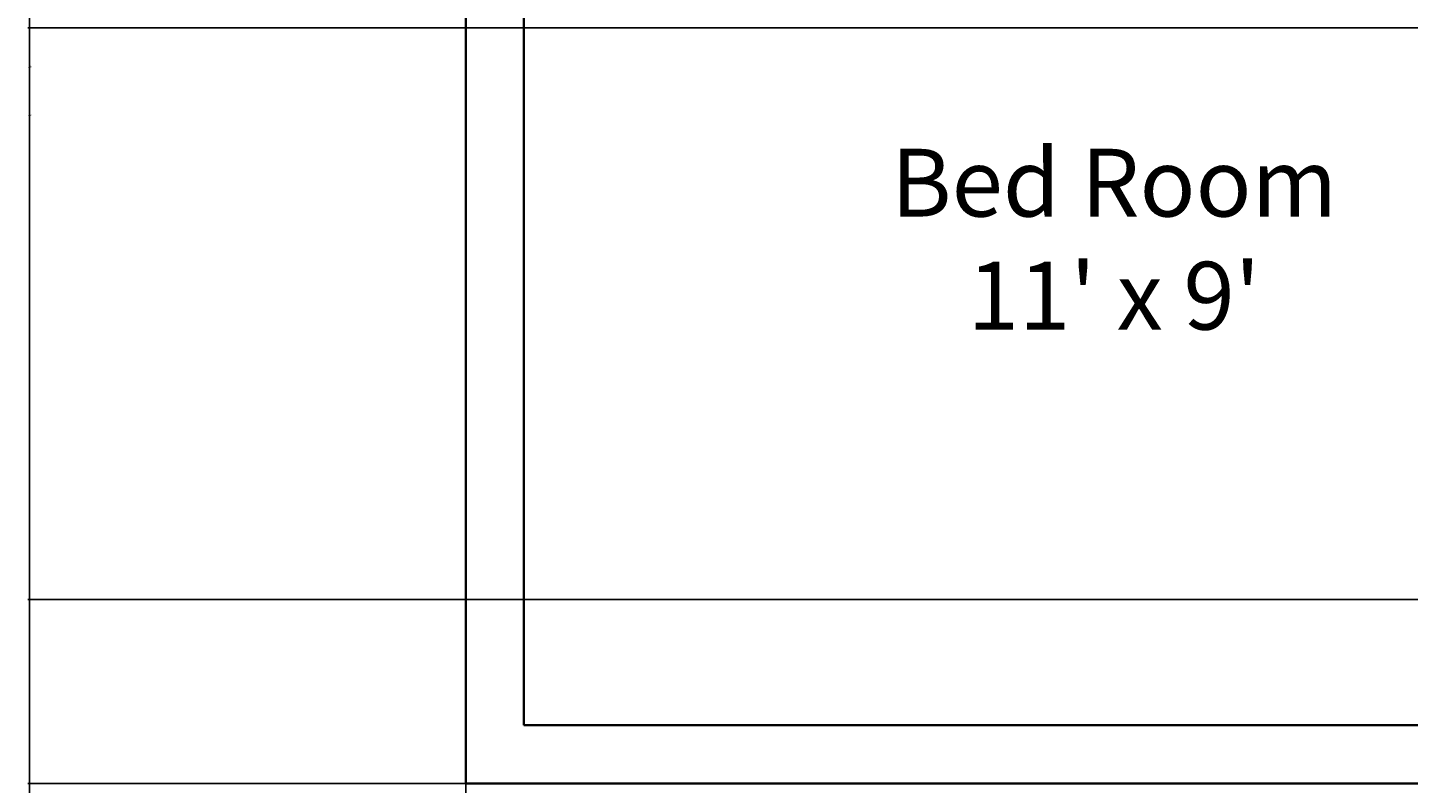
# Model space of a CAD drawing. Units: feet. Extents: x 105 to 1094, y -88 to 588.
# Tile 5 of 59: x 105 to 248, y 276 to 354. Entities that reach past the tile are written whole.
import ezdxf

# ---------------------------------------------------------------- set-up
doc = ezdxf.new("R2010")
doc.units = ezdxf.units.FT
doc.header["$MEASUREMENT"] = 0
for name, color, linetype, lineweight in [('A-ANNO-DIMS', 2, 'Continuous', 18), ('A-AREA-IDEN', 7, 'Continuous', 18), ('A-WALL', 7, 'Continuous', 35)]:
    doc.layers.add(name, color=color, linetype=linetype, lineweight=lineweight)
doc.styles.get("Standard").update_dxf_attribs({"font": 'arial.ttf'})
doc.dimstyles.get("Standard").update_dxf_attribs({"dimtxt": 0.18, "dimasz": 0.18, "dimexe": 0.18, "dimexo": 0.0625, "dimgap": 0.09, "dimtad": 0, "dimtih": 1, "dimtoh": 1, "dimdec": 4, "dimzin": 0, "dimdsep": 46, "dimtxsty": 'Standard', "dimcen": 0.09, "dimadec": 0, "dimazin": 0, "dimtfac": 1, "dimtdec": 4, "dimtofl": 0, "dimtmove": 0, "dimatfit": 3, "dimfxl": 1, "dimtolj": 1, "dimtzin": 0, "dimarcsym": 0})

# ---------------------------------------------------------------- blocks, each defined once
blk = doc.blocks.new('*D21')
at = {"layer": 'A-ANNO-DIMS', "color": 0, "lineweight": -2, "transparency": 16777216}
for p, q in [((849.63, 543.08), (105.46, 543.08)), ((105.64, 542.9), (105.64, 250.26)), ((105.64, -42.74), (105.64, 249.9)), ((849.63, -42.92), (105.46, -42.92))]:
    blk.add_line(p, q, dxfattribs=at)
at = {"layer": 'A-ANNO-DIMS', "color": 0, "transparency": 16777216}
for points in [[(105.61, 542.9), (105.67, 542.9), (105.64, 543.08)], [(105.61, -42.74), (105.67, -42.74), (105.64, -42.92)]]:
    blk.add_solid(points, dxfattribs=at)
at = {"layer": 'Defpoints', "color": 0, "transparency": 16777216}
for p in [(105.64, 543.08), (849.69, 543.08), (849.69, -42.92)]:
    blk.add_point(p, dxfattribs=at)
at = {"layer": 'A-ANNO-DIMS', "color": 0, "transparency": 16777216, "insert": (105.64, 250.08), "char_height": 0.18, "attachment_point": 5}
blk.add_mtext('\\A1;586', dxfattribs=at)
blk = doc.blocks.new('*D28')
at = {"layer": 'A-ANNO-DIMS', "color": 0, "lineweight": -2, "transparency": 16777216}
for p, q in [((150.63, 424.08), (105.46, 424.08)), ((105.64, 423.9), (105.64, 350.26)), ((105.64, 276.26), (105.64, 349.9)), ((150.63, 276.08), (105.46, 276.08))]:
    blk.add_line(p, q, dxfattribs=at)
at = {"layer": 'A-ANNO-DIMS', "color": 0, "transparency": 16777216}
for points in [[(105.61, 423.9), (105.67, 423.9), (105.64, 424.08)], [(105.61, 276.26), (105.67, 276.26), (105.64, 276.08)]]:
    blk.add_solid(points, dxfattribs=at)
at = {"layer": 'Defpoints', "color": 0, "transparency": 16777216}
for p in [(105.64, 424.08), (150.69, 424.08), (150.69, 276.08)]:
    blk.add_point(p, dxfattribs=at)
at = {"layer": 'A-ANNO-DIMS', "color": 0, "transparency": 16777216, "insert": (105.64, 350.08), "char_height": 0.18, "attachment_point": 5}
blk.add_mtext('\\A1;148', dxfattribs=at)
blk = doc.blocks.new('*D33')
at = {"layer": 'A-ANNO-DIMS', "color": 0, "lineweight": -2, "transparency": 16777216}
for p, q in [((646.63, 395.08), (105.46, 395.08)), ((105.64, 394.9), (105.64, 345.26)), ((105.64, 295.26), (105.64, 344.9)), ((646.63, 295.08), (105.46, 295.08))]:
    blk.add_line(p, q, dxfattribs=at)
at = {"layer": 'A-ANNO-DIMS', "color": 0, "transparency": 16777216}
for points in [[(105.61, 394.9), (105.67, 394.9), (105.64, 395.08)], [(105.61, 295.26), (105.67, 295.26), (105.64, 295.08)]]:
    blk.add_solid(points, dxfattribs=at)
at = {"layer": 'Defpoints', "color": 0, "transparency": 16777216}
for p in [(646.69, 395.08), (105.64, 295.08), (646.69, 295.08)]:
    blk.add_point(p, dxfattribs=at)
at = {"layer": 'A-ANNO-DIMS', "color": 0, "transparency": 16777216, "insert": (105.64, 345.08), "char_height": 0.18, "attachment_point": 5}
blk.add_mtext('\\A1;100', dxfattribs=at)
blk = doc.blocks.new('*D38')
at = {"layer": 'A-ANNO-DIMS', "color": 0, "lineweight": -2, "transparency": 16777216}
for p, q in [((150.69, 224.14), (150.69, 588.31)), ((150.87, 588.13), (222.41, 588.13)), ((294.51, 588.13), (222.97, 588.13)), ((294.69, 224.14), (294.69, 588.31))]:
    blk.add_line(p, q, dxfattribs=at)
at = {"layer": 'A-ANNO-DIMS', "color": 0, "transparency": 16777216}
for points in [[(150.87, 588.16), (150.87, 588.1), (150.69, 588.13)], [(294.51, 588.16), (294.51, 588.1), (294.69, 588.13)]]:
    blk.add_solid(points, dxfattribs=at)
at = {"layer": 'Defpoints', "color": 0, "transparency": 16777216}
for p in [(294.69, 588.13), (150.69, 224.08), (294.69, 224.08)]:
    blk.add_point(p, dxfattribs=at)
at = {"layer": 'A-ANNO-DIMS', "color": 0, "transparency": 16777216, "insert": (222.69, 588.13), "char_height": 0.18, "attachment_point": 5}
blk.add_mtext('\\A1;144', dxfattribs=at)
blk = doc.blocks.new('*D51')
at = {"layer": 'A-ANNO-DIMS', "color": 0, "lineweight": -2, "transparency": 16777216}
for p, q in [((432.63, 394.08), (105.46, 394.08)), ((105.64, 393.9), (105.64, 374.26)), ((105.64, 354.26), (105.64, 373.9)), ((426.63, 354.08), (105.46, 354.08))]:
    blk.add_line(p, q, dxfattribs=at)
at = {"layer": 'A-ANNO-DIMS', "color": 0, "transparency": 16777216}
for points in [[(105.61, 393.9), (105.67, 393.9), (105.64, 394.08)], [(105.61, 354.26), (105.67, 354.26), (105.64, 354.08)]]:
    blk.add_solid(points, dxfattribs=at)
at = {"layer": 'Defpoints', "color": 0, "transparency": 16777216}
for p in [(432.69, 394.08), (105.64, 354.08), (426.69, 354.08)]:
    blk.add_point(p, dxfattribs=at)
at = {"layer": 'A-ANNO-DIMS', "color": 0, "transparency": 16777216, "insert": (105.64, 374.08), "char_height": 0.18, "attachment_point": 5}
blk.add_mtext('\\A1;40', dxfattribs=at)

msp = doc.modelspace()

# ---------------------------------------------------------------- linework, layer by layer
at = {"layer": 'A-WALL'}
for p, q in [((150.6883, 276.0812), (150.6883, 394.0812)), ((156.6883, 282.0812), (156.6883, 390.0812)), ((288.6883, 282.0812), (156.6883, 282.0812)), ((294.6883, 276.0812), (150.6883, 276.0812))]:
    msp.add_line(p, q, dxfattribs=at)

# ---------------------------------------------------------------- texts
at = {"layer": 'A-AREA-IDEN', "insert": (266.8257, 341.6038), "char_height": 7, "attachment_point": 3}
msp.add_mtext_dynamic_manual_height_columns("\\pxqc;Bed Room \\P11' x 9'", width=98.34246, gutter_width=1, heights=[0], dxfattribs=at)

# ---------------------------------------------------------------- dimensions: what is measured, and where the dimension line sits
at = {"layer": 'A-ANNO-DIMS'}
dim = msp.add_linear_dim(base=(294.6883, 588.1312), p1=(150.6883, 224.0812), p2=(294.6883, 224.0812), dimstyle='Standard', override={"dimdec": 0, "dimlfac": 1, "dimrnd": 0, "dimzin": 0, "dimdsep": 46, "dimlunit": 2}, dxfattribs=at)
dim.commit()
dim.dimension.update_dxf_attribs({"geometry": '*D38', "text_midpoint": (222.6883, 588.1312)})
for base, p1, p2, picture, middle in [((105.6383, 543.0812), (849.6883, -42.9188), (849.6883, 543.0812), '*D21', (105.6383, 250.0812)), ((105.6383, 424.0812), (150.6883, 276.0812), (150.6883, 424.0812), '*D28', (105.6383, 350.0812)), ((105.6383, 295.0812), (646.6883, 395.0812), (646.6883, 295.0812), '*D33', (105.6383, 345.0812)), ((105.6383, 354.0812), (432.6883, 394.0812), (426.6883, 354.0812), '*D51', (105.6383, 374.0812))]:
    dim = msp.add_linear_dim(base=base, p1=p1, p2=p2, angle=90, dimstyle='Standard', override={"dimdec": 0, "dimlfac": 1, "dimrnd": 0, "dimzin": 0, "dimdsep": 46, "dimlunit": 2}, dxfattribs=at)
    dim.commit()
    dim.dimension.update_dxf_attribs({"geometry": picture, "text_midpoint": middle})

doc.saveas('drawing.dxf')
